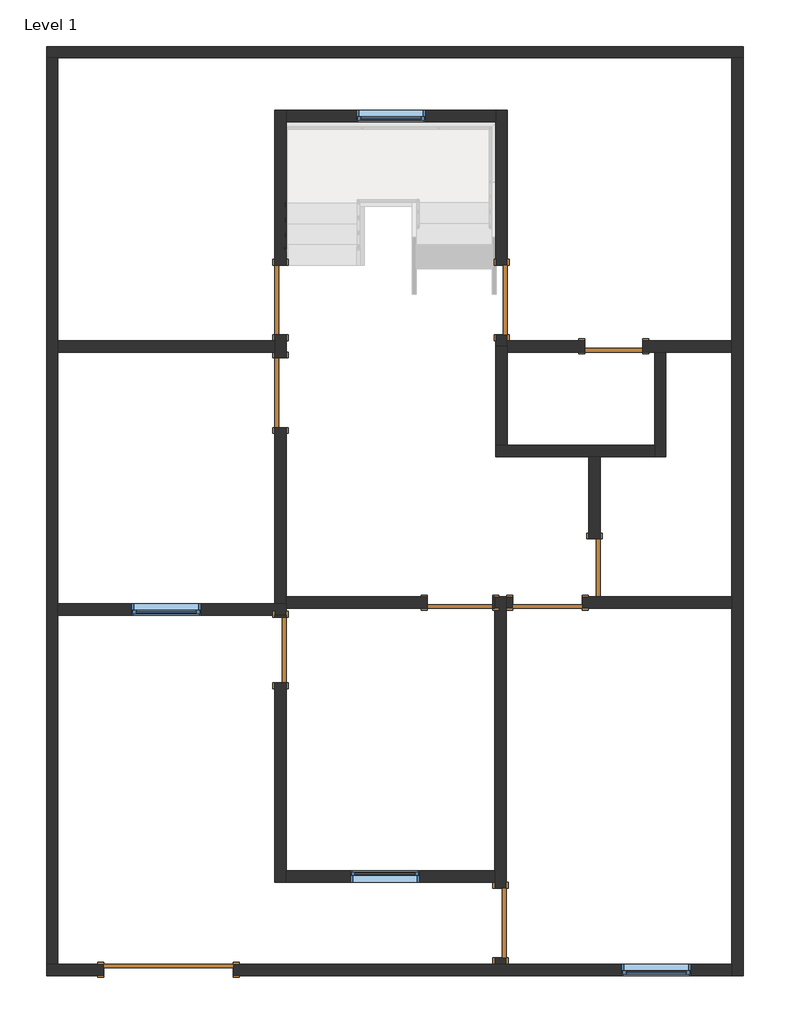
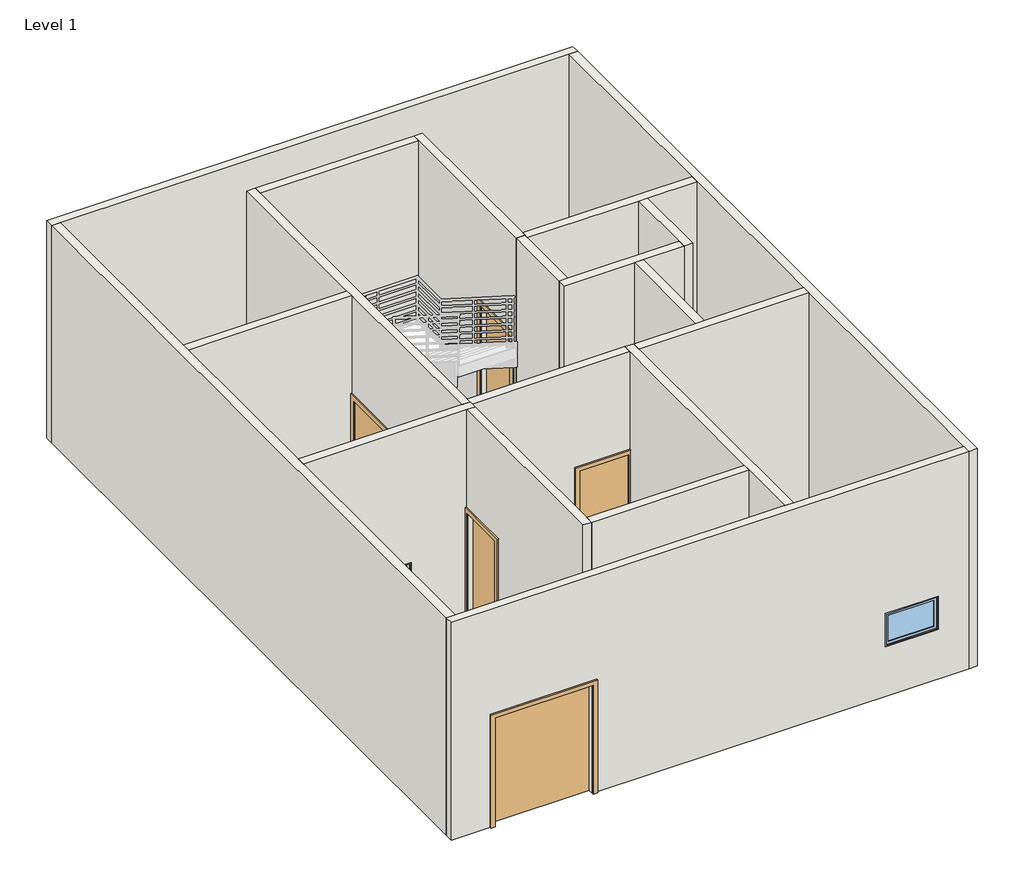
# One storey, part 1 of 3: 19 walls, 10 doors, 4 windows.
"""IFC4 building model written with IfcOpenShell, lengths in millimetres."""

from ifc_helpers import new_model, si_unit, frame, origin, origin_with_axes, place, context, project, spatial, polyline, outline, extrude, faceted_brep, transform, mapped, element, save
from components import m_door_double_flush_panel_double_acting_1700_x_2000mm_42eec5da, m_single_flush_0762_x_2032mm_ffa3ef71, m_single_flush_0762_x_2032mm_3f592dcc, m_single_flush_0864_x_2134mm_0748c0c9, m_single_flush_0915_x_2032mm_d0c19338, m_single_flush_0915_x_2134mm_f3d7f739, m_single_flush_0915_x_2134mm_138fd904, m_fixed_0915_x_0610mm_ad787ded

model = new_model("IFC4")

# Units and contexts
model_context = context("Model", 3, world=origin())
ifc_project = project(units=[si_unit("LENGTHUNIT", "METRE", prefix="MILLI")], contexts=[model_context])

# Site, building, storey
site = spatial("IfcSite", under=ifc_project)
building = spatial("IfcBuilding", under=site)
storey = spatial("IfcBuildingStorey", under=building, Name="Level 1", Elevation=0.0)

# Doors
placement = place(None, origin())
m_door_double_flush_panel_double_acting_1700_x_2000mm_shape = m_door_double_flush_panel_double_acting_1700_x_2000mm_42eec5da(model_context)
element("IfcDoor", 1, ObjectType="M_Door-Double-Flush_Panel-Double-Acting : 1700 x 2000mm", at=placement, inside=storey, context=model_context, shape_type="MappedRepresentation", body=[
    mapped(m_door_double_flush_panel_double_acting_1700_x_2000mm_shape, transform((-12117.6012725, -246.6487671, 0.0), x_axis=(1.0, 0.0, 0.0), y_axis=(0.0, 1.0, 0.0), z_axis=(0.0, 0.0, 1.0))),
])
m_single_flush_0762_x_2032mm_shape = m_single_flush_0762_x_2032mm_ffa3ef71(model_context)
element("IfcDoor", 2, ObjectType="M_Single-Flush : 0762 x 2032mm", at=placement, inside=storey, context=model_context, shape_type="MappedRepresentation", body=[
    mapped(m_single_flush_0762_x_2032mm_shape, transform((-6272.0012725, 7935.7512329, 0.0), x_axis=(1.0, 0.0, 0.0), y_axis=(0.0, 1.0, 0.0), z_axis=(0.0, 0.0, 1.0))),
])
m_single_flush_0762_x_2032mm_2_shape = m_single_flush_0762_x_2032mm_3f592dcc(model_context)
element("IfcDoor", 3, ObjectType="M_Single-Flush : 0762 x 2032mm", at=placement, inside=storey, context=model_context, shape_type="MappedRepresentation", body=[
    mapped(m_single_flush_0762_x_2032mm_2_shape, transform((-6526.0012725, 5028.6512329, 0.0), x_axis=(0.0, -1.0, 0.0), y_axis=(1.0, 0.0, 0.0), z_axis=(0.0, 0.0, 1.0))),
])
m_single_flush_0864_x_2134mm_shape = m_single_flush_0864_x_2134mm_0748c0c9(model_context)
element("IfcDoor", 4, ObjectType="M_Single-Flush : 0864 x 2134mm", at=placement, inside=storey, context=model_context, shape_type="MappedRepresentation", body=[
    mapped(m_single_flush_0864_x_2134mm_shape, transform((-10646.8012725, 3950.3512329, 0.0), x_axis=(0.0, 1.0, 0.0), y_axis=(-1.0, 0.0, 0.0), z_axis=(0.0, 0.0, 1.0))),
])
element("IfcDoor", 5, ObjectType="M_Single-Flush : 0864 x 2134mm", at=placement, inside=storey, context=model_context, shape_type="MappedRepresentation", body=[
    mapped(m_single_flush_0864_x_2134mm_shape, transform((-8290.1012725, 4571.4512329, 0.0), x_axis=(1.0, 0.0, 0.0), y_axis=(0.0, 1.0, 0.0), z_axis=(0.0, 0.0, 1.0))),
])
m_single_flush_0915_x_2032mm_shape = m_single_flush_0915_x_2032mm_d0c19338(model_context)
element("IfcDoor", 6, ObjectType="M_Single-Flush : 0915 x 2032mm", at=placement, inside=storey, context=model_context, shape_type="MappedRepresentation", body=[
    mapped(m_single_flush_0915_x_2032mm_shape, transform((-7141.9512725, 4571.4512329, 0.0), x_axis=(-1.0, 0.0, 0.0), y_axis=(0.0, -1.0, 0.0), z_axis=(0.0, 0.0, 1.0))),
])
element("IfcDoor", 7, ObjectType="M_Single-Flush : 0915 x 2032mm", at=placement, inside=storey, context=model_context, shape_type="MappedRepresentation", body=[
    mapped(m_single_flush_0915_x_2032mm_shape, transform((-7757.9012725, 366.5512329, 0.0), x_axis=(0.0, -1.0, 0.0), y_axis=(1.0, 0.0, 0.0), z_axis=(0.0, 0.0, 1.0))),
])
m_single_flush_0915_x_2134mm_shape = m_single_flush_0915_x_2134mm_f3d7f739(model_context)
element("IfcDoor", 8, ObjectType="M_Single-Flush : 0915 x 2134mm", at=placement, inside=storey, context=model_context, shape_type="MappedRepresentation", body=[
    mapped(m_single_flush_0915_x_2134mm_shape, transform((-10646.8012725, 8545.3512329, 0.0), x_axis=(0.0, -1.0, 0.0), y_axis=(1.0, 0.0, 0.0), z_axis=(0.0, 0.0, 1.0))),
])
m_single_flush_0915_x_2134mm_2_shape = m_single_flush_0915_x_2134mm_138fd904(model_context)
element("IfcDoor", 9, ObjectType="M_Single-Flush : 0915 x 2134mm", at=placement, inside=storey, context=model_context, shape_type="MappedRepresentation", body=[
    mapped(m_single_flush_0915_x_2134mm_2_shape, transform((-7744.0012725, 8545.3512329, 0.0), x_axis=(0.0, -1.0, 0.0), y_axis=(1.0, 0.0, 0.0), z_axis=(0.0, 0.0, 1.0))),
])
element("IfcDoor", 10, ObjectType="M_Single-Flush : 0915 x 2134mm", at=placement, inside=storey, context=model_context, shape_type="MappedRepresentation", body=[
    mapped(m_single_flush_0915_x_2134mm_2_shape, transform((-10646.8012725, 7326.1512329, 0.0), x_axis=(0.0, 1.0, 0.0), y_axis=(-1.0, 0.0, 0.0), z_axis=(0.0, 0.0, 1.0))),
])

# Walls
element("IfcWall", 11, ObjectType="Generic - 150mm", at=placement, inside=storey, context=model_context, shape_type="Brep", body=[
    faceted_brep([(-13716.6012725, 11720.3512329, 0.0), (-13566.6012725, 11720.3512329, 0.0), (-4722.6012725, 11720.3512329, 0.0), (-4572.6012725, 11720.3512329, 0.0), (-4572.6012725, 11720.3512329, 4000.0), (-4722.6012725, 11720.3512329, 4000.0), (-13566.6012725, 11720.3512329, 4000.0), (-13716.6012725, 11720.3512329, 4000.0), (-13716.6012725, 11870.3512329, 0.0), (-13716.6012725, 11870.3512329, 4000.0), (-4572.6012725, 11870.3512329, 4000.0), (-4572.6012725, 11870.3512329, 0.0)], [[[0, 1, 2, 3, 4, 5, 6, 7]], [[8, 9, 10, 11]], [[3, 2, 1, 0, 8, 11]], [[7, 6, 5, 4, 10, 9]], [[4, 3, 11, 10]], [[0, 7, 9, 8]]]),
])
element("IfcWall", 12, ObjectType="Generic - 150mm", at=placement, inside=storey, context=model_context, shape_type="Brep", body=[
    faceted_brep([(-4722.6012725, 11720.3512329, 0.0), (-4722.6012725, 8010.7512329, 0.0), (-4722.6012725, 7860.7512329, 0.0), (-4722.6012725, 4646.4512329, 0.0), (-4722.6012725, 4496.4512329, 0.0), (-4722.6012725, -171.6487671, 0.0), (-4722.6012725, -321.6487671, 0.0), (-4722.6012725, -321.6487671, 4000.0), (-4722.6012725, -171.6487671, 4000.0), (-4722.6012725, 4496.4512329, 4000.0), (-4722.6012725, 4646.4512329, 4000.0), (-4722.6012725, 7860.7512329, 4000.0), (-4722.6012725, 8010.7512329, 4000.0), (-4722.6012725, 11720.3512329, 4000.0), (-4572.6012725, 11720.3512329, 0.0), (-4572.6012725, 11720.3512329, 4000.0), (-4572.6012725, -321.6487671, 4000.0), (-4572.6012725, -321.6487671, 0.0)], [[[0, 1, 2, 3, 4, 5, 6, 7, 8, 9, 10, 11, 12, 13]], [[14, 15, 16, 17]], [[6, 5, 4, 3, 2, 1, 0, 14, 17]], [[13, 12, 11, 10, 9, 8, 7, 16, 15]], [[0, 13, 15, 14]], [[7, 6, 17, 16]]]),
])
element("IfcWall", 13, ObjectType="Generic - 150mm", at=placement, inside=storey, context=model_context, shape_type="Brep", body=[
    faceted_brep([(-13716.6012725, -171.6487671, 4000.0), (-13566.6012725, -171.6487671, 4000.0), (-7832.9012725, -171.6487671, 4000.0), (-7682.9012725, -171.6487671, 4000.0), (-4722.6012725, -171.6487671, 4000.0), (-4722.6012725, -171.6487671, 0.0), (-7682.9012725, -171.6487671, 0.0), (-7832.9012725, -171.6487671, 0.0), (-11267.6012725, -171.6487671, 0.0), (-11267.6012725, -171.6487671, 2000.0), (-12967.6012725, -171.6487671, 2000.0), (-12967.6012725, -171.6487671, 0.0), (-13566.6012725, -171.6487671, 0.0), (-13716.6012725, -171.6487671, 0.0), (-5256.9012725, -171.6487671, 915.0), (-5256.9012725, -171.6487671, 1525.0), (-6171.9012725, -171.6487671, 1525.0), (-6171.9012725, -171.6487671, 915.0), (-4722.6012725, -321.6487671, 4000.0), (-13716.6012725, -321.6487671, 4000.0), (-13716.6012725, -321.6487671, 0.0), (-12967.6012725, -321.6487671, 0.0), (-12967.6012725, -321.6487671, 2000.0), (-11267.6012725, -321.6487671, 2000.0), (-11267.6012725, -321.6487671, 0.0), (-4722.6012725, -321.6487671, 0.0), (-5256.9012725, -321.6487671, 915.0), (-6171.9012725, -321.6487671, 915.0), (-6171.9012725, -321.6487671, 1525.0), (-5256.9012725, -321.6487671, 1525.0)], [[[0, 1, 2, 3, 4, 5, 6, 7, 8, 9, 10, 11, 12, 13], [14, 15, 16, 17]], [[18, 19, 20, 21, 22, 23, 24, 25], [26, 27, 28, 29]], [[5, 25, 24, 8, 7, 6]], [[20, 13, 12, 11, 21]], [[4, 3, 2, 1, 0, 19, 18]], [[5, 4, 18, 25]], [[0, 13, 20, 19]], [[23, 9, 8, 24]], [[9, 23, 22, 10]], [[10, 22, 21, 11]], [[15, 14, 26, 29]], [[16, 15, 29, 28]], [[17, 16, 28, 27]], [[14, 17, 27, 26]]]),
])
element("IfcWall", 14, ObjectType="Generic - 150mm", at=placement, inside=storey, context=model_context, shape_type="Brep", body=[
    faceted_brep([(-13566.6012725, -171.6487671, 0.0), (-13566.6012725, 4407.5512329, 0.0), (-13566.6012725, 4557.5512329, 0.0), (-13566.6012725, 7860.7512329, 0.0), (-13566.6012725, 8010.7512329, 0.0), (-13566.6012725, 11720.3512329, 0.0), (-13566.6012725, 11720.3512329, 4000.0), (-13566.6012725, 8010.7512329, 4000.0), (-13566.6012725, 7860.7512329, 4000.0), (-13566.6012725, 4557.5512329, 4000.0), (-13566.6012725, 4407.5512329, 4000.0), (-13566.6012725, -171.6487671, 4000.0), (-13716.6012725, -171.6487671, 0.0), (-13716.6012725, -171.6487671, 4000.0), (-13716.6012725, 11720.3512329, 4000.0), (-13716.6012725, 11720.3512329, 0.0)], [[[0, 1, 2, 3, 4, 5, 6, 7, 8, 9, 10, 11]], [[12, 13, 14, 15]], [[5, 4, 3, 2, 1, 0, 12, 15]], [[11, 10, 9, 8, 7, 6, 14, 13]], [[6, 5, 15, 14]], [[0, 11, 13, 12]]]),
])
element("IfcWall", 15, ObjectType="Generic - 150mm", at=placement, inside=storey, context=model_context, shape_type="SweptSolid", body=[
    extrude(outline(polyline([(-10721.8012725, 7860.7512329), (-13566.6012725, 7860.7512329), (-13566.6012725, 8010.7512329), (-10721.8012725, 8010.7512329), (-10721.8012725, 7860.7512329)])), origin_with_axes(), (0.0, 0.0, 1.0), 4000.0),
])
element("IfcWall", 16, ObjectType="Generic - 150mm", at=placement, inside=storey, context=model_context, shape_type="Brep", body=[
    faceted_brep([(-10571.8012725, 7783.6512329, 2134.0), (-10571.8012725, 7783.6512329, 0.0), (-10571.8012725, 8087.8512329, 0.0), (-10571.8012725, 8087.8512329, 2134.0), (-10571.8012725, 9002.8512329, 2134.0), (-10571.8012725, 9002.8512329, 0.0), (-10571.8012725, 10883.3512329, 0.0), (-10571.8012725, 11033.3512329, 0.0), (-10571.8012725, 11033.3512329, 4000.0), (-10571.8012725, 10883.3512329, 4000.0), (-10571.8012725, 4646.4512329, 4000.0), (-10571.8012725, 4557.5512329, 4000.0), (-10571.8012725, 4557.5512329, 0.0), (-10571.8012725, 4646.4512329, 0.0), (-10571.8012725, 6868.6512329, 0.0), (-10571.8012725, 6868.6512329, 2134.0), (-10721.8012725, 8087.8512329, 0.0), (-10721.8012725, 8010.7512329, 0.0), (-10721.8012725, 7860.7512329, 0.0), (-10721.8012725, 7783.6512329, 0.0), (-10721.8012725, 7783.6512329, 2134.0), (-10721.8012725, 6868.6512329, 2134.0), (-10721.8012725, 6868.6512329, 0.0), (-10721.8012725, 4557.5512329, 0.0), (-10721.8012725, 4557.5512329, 4000.0), (-10721.8012725, 7860.7512329, 4000.0), (-10721.8012725, 8010.7512329, 4000.0), (-10721.8012725, 11033.3512329, 4000.0), (-10721.8012725, 11033.3512329, 0.0), (-10721.8012725, 9002.8512329, 0.0), (-10721.8012725, 9002.8512329, 2134.0), (-10721.8012725, 8087.8512329, 2134.0)], [[[0, 1, 2, 3, 4, 5, 6, 7, 8, 9, 10, 11, 12, 13, 14, 15]], [[16, 17, 18, 19, 20, 21, 22, 23, 24, 25, 26, 27, 28, 29, 30, 31]], [[29, 28, 7, 6, 5]], [[2, 1, 19, 18, 17, 16]], [[14, 13, 12, 23, 22]], [[11, 10, 9, 8, 27, 26, 25, 24]], [[12, 11, 24, 23]], [[3, 2, 16, 31]], [[4, 3, 31, 30]], [[5, 4, 30, 29]], [[20, 19, 1, 0]], [[21, 20, 0, 15]], [[22, 21, 15, 14]], [[8, 7, 28, 27]]]),
])
element("IfcWall", 17, ObjectType="Generic - 150mm", at=placement, inside=storey, context=model_context, shape_type="Brep", body=[
    faceted_brep([(-4722.6012725, 8010.7512329, 0.0), (-5891.0012725, 8010.7512329, 0.0), (-5891.0012725, 8010.7512329, 2032.0), (-6653.0012725, 8010.7512329, 2032.0), (-6653.0012725, 8010.7512329, 0.0), (-7669.0012725, 8010.7512329, 0.0), (-7669.0012725, 8010.7512329, 4000.0), (-4722.6012725, 8010.7512329, 4000.0), (-5891.0012725, 7860.7512329, 2032.0), (-5891.0012725, 7860.7512329, 0.0), (-5737.4012725, 7860.7512329, 0.0), (-5587.4012725, 7860.7512329, 0.0), (-4722.6012725, 7860.7512329, 0.0), (-4722.6012725, 7860.7512329, 4000.0), (-5587.4012725, 7860.7512329, 4000.0), (-5737.4012725, 7860.7512329, 4000.0), (-7672.6012725, 7860.7512329, 4000.0), (-7672.6012725, 7860.7512329, 0.0), (-6653.0012725, 7860.7512329, 0.0), (-6653.0012725, 7860.7512329, 2032.0), (-7672.6012725, 7935.7512329, 0.0), (-7669.0012725, 7935.7512329, 0.0), (-7669.0012725, 7935.7512329, 4000.0), (-7672.6012725, 7935.7512329, 4000.0)], [[[0, 1, 2, 3, 4, 5, 6, 7]], [[8, 9, 10, 11, 12, 13, 14, 15, 16, 17, 18, 19]], [[18, 17, 20, 21, 5, 4]], [[12, 11, 10, 9, 1, 0]], [[7, 6, 22, 23, 16, 15, 14, 13]], [[0, 7, 13, 12]], [[6, 5, 21, 22]], [[21, 20, 23, 22]], [[20, 17, 16, 23]], [[2, 1, 9, 8]], [[3, 2, 8, 19]], [[4, 3, 19, 18]]]),
])
element("IfcWall", 18, ObjectType="Generic - 150mm", at=placement, inside=storey, context=model_context, shape_type="Brep", body=[
    faceted_brep([(-7669.0012725, 7935.7512329, 0.0), (-7669.0012725, 8010.7512329, 0.0), (-7669.0012725, 8087.8512329, 0.0), (-7669.0012725, 8087.8512329, 2134.0), (-7669.0012725, 9002.8512329, 2134.0), (-7669.0012725, 9002.8512329, 0.0), (-7669.0012725, 11033.3512329, 0.0), (-7669.0012725, 11033.3512329, 4000.0), (-7669.0012725, 8010.7512329, 4000.0), (-7669.0012725, 7935.7512329, 4000.0), (-7819.0012725, 8087.8512329, 2134.0), (-7819.0012725, 8087.8512329, 0.0), (-7819.0012725, 7935.7512329, 0.0), (-7819.0012725, 7935.7512329, 4000.0), (-7819.0012725, 10883.3512329, 4000.0), (-7819.0012725, 11033.3512329, 4000.0), (-7819.0012725, 11033.3512329, 0.0), (-7819.0012725, 10883.3512329, 0.0), (-7819.0012725, 9002.8512329, 0.0), (-7819.0012725, 9002.8512329, 2134.0), (-7672.6012725, 7935.7512329, 0.0), (-7672.6012725, 7935.7512329, 4000.0)], [[[0, 1, 2, 3, 4, 5, 6, 7, 8, 9]], [[10, 11, 12, 13, 14, 15, 16, 17, 18, 19]], [[12, 11, 2, 1, 0, 20]], [[18, 17, 16, 6, 5]], [[9, 8, 7, 15, 14, 13, 21]], [[0, 9, 21, 13, 12, 20]], [[3, 2, 11, 10]], [[4, 3, 10, 19]], [[5, 4, 19, 18]], [[7, 6, 16, 15]]]),
])
element("IfcWall", 19, ObjectType="Generic - 150mm", at=placement, inside=storey, context=model_context, shape_type="Brep", body=[
    faceted_brep([(-13566.6012725, 4407.5512329, 0.0), (-10721.8012725, 4407.5512329, 0.0), (-10571.8012725, 4407.5512329, 0.0), (-10571.8012725, 4407.5512329, 4000.0), (-10721.8012725, 4407.5512329, 4000.0), (-13566.6012725, 4407.5512329, 4000.0), (-11686.7012725, 4407.5512329, 915.0), (-12601.7012725, 4407.5512329, 915.0), (-12601.7012725, 4407.5512329, 1525.0), (-11686.7012725, 4407.5512329, 1525.0), (-13566.6012725, 4557.5512329, 0.0), (-13566.6012725, 4557.5512329, 4000.0), (-10721.8012725, 4557.5512329, 4000.0), (-10571.8012725, 4557.5512329, 4000.0), (-10571.8012725, 4557.5512329, 0.0), (-10721.8012725, 4557.5512329, 0.0), (-11686.7012725, 4557.5512329, 915.0), (-11686.7012725, 4557.5512329, 1525.0), (-12601.7012725, 4557.5512329, 1525.0), (-12601.7012725, 4557.5512329, 915.0), (-10571.8012725, 4496.4512329, 0.0), (-10571.8012725, 4496.4512329, 4000.0)], [[[0, 1, 2, 3, 4, 5], [6, 7, 8, 9]], [[10, 11, 12, 13, 14, 15], [16, 17, 18, 19]], [[2, 1, 0, 10, 15, 14, 20]], [[5, 4, 3, 21, 13, 12, 11]], [[0, 5, 11, 10]], [[3, 2, 20, 14, 13, 21]], [[17, 16, 6, 9]], [[18, 17, 9, 8]], [[19, 18, 8, 7]], [[16, 19, 7, 6]]]),
])
element("IfcWall", 20, ObjectType="Generic - 150mm", at=placement, inside=storey, context=model_context, shape_type="Brep", body=[
    faceted_brep([(-5737.4012725, 7860.7512329, 0.0), (-5737.4012725, 6639.1512329, 0.0), (-5737.4012725, 6489.1512329, 0.0), (-5737.4012725, 6489.1512329, 4000.0), (-5737.4012725, 6639.1512329, 4000.0), (-5737.4012725, 7860.7512329, 4000.0), (-5587.4012725, 7860.7512329, 0.0), (-5587.4012725, 7860.7512329, 4000.0), (-5587.4012725, 6489.1512329, 4000.0), (-5587.4012725, 6489.1512329, 0.0)], [[[0, 1, 2, 3, 4, 5]], [[6, 7, 8, 9]], [[2, 1, 0, 6, 9]], [[5, 4, 3, 8, 7]], [[0, 5, 7, 6]], [[3, 2, 9, 8]]]),
])
element("IfcWall", 21, ObjectType="Generic - 150mm", at=placement, inside=storey, context=model_context, shape_type="Brep", body=[
    faceted_brep([(-5737.4012725, 6639.1512329, 0.0), (-7672.6012725, 6639.1512329, 0.0), (-7822.6012725, 6639.1512329, 0.0), (-7822.6012725, 6639.1512329, 4000.0), (-7672.6012725, 6639.1512329, 4000.0), (-5737.4012725, 6639.1512329, 4000.0), (-5737.4012725, 6489.1512329, 0.0), (-5737.4012725, 6489.1512329, 4000.0), (-6451.0012725, 6489.1512329, 4000.0), (-6601.0012725, 6489.1512329, 4000.0), (-7822.6012725, 6489.1512329, 4000.0), (-7822.6012725, 6489.1512329, 0.0), (-6601.0012725, 6489.1512329, 0.0), (-6451.0012725, 6489.1512329, 0.0)], [[[0, 1, 2, 3, 4, 5]], [[6, 7, 8, 9, 10, 11, 12, 13]], [[2, 1, 0, 6, 13, 12, 11]], [[5, 4, 3, 10, 9, 8, 7]], [[0, 5, 7, 6]], [[3, 2, 11, 10]]]),
])
element("IfcWall", 22, ObjectType="Generic - 150mm", at=placement, inside=storey, context=model_context, shape_type="Brep", body=[
    faceted_brep([(-7672.6012725, 6639.1512329, 0.0), (-7672.6012725, 7860.7512329, 0.0), (-7672.6012725, 7935.7512329, 0.0), (-7672.6012725, 7935.7512329, 4000.0), (-7672.6012725, 7860.7512329, 4000.0), (-7672.6012725, 6639.1512329, 4000.0), (-7822.6012725, 6639.1512329, 0.0), (-7822.6012725, 6639.1512329, 4000.0), (-7822.6012725, 7935.7512329, 4000.0), (-7822.6012725, 7935.7512329, 0.0), (-7819.0012725, 7935.7512329, 0.0), (-7819.0012725, 7935.7512329, 4000.0)], [[[0, 1, 2, 3, 4, 5]], [[6, 7, 8, 9]], [[2, 1, 0, 6, 9, 10]], [[3, 2, 10, 9, 8, 11]], [[5, 4, 3, 11, 8, 7]], [[0, 5, 7, 6]]]),
])
element("IfcWall", 23, ObjectType="Generic - 150mm", at=placement, inside=storey, context=model_context, shape_type="SweptSolid", body=[
    extrude(outline(polyline([(4647.6512329, 2032.0), (4647.6512329, 0.0), (4646.4512329, 0.0), (4646.4512329, 4000.0), (6489.1512329, 4000.0), (6489.1512329, 0.0), (5409.6512329, 0.0), (5409.6512329, 2032.0), (4647.6512329, 2032.0)])), frame((-6601.0012725, 0.0, 0.0), z_axis=(1.0, 0.0, 0.0), x_axis=(0.0, 1.0, 0.0)), (0.0, 0.0, 1.0), 150.0),
])
element("IfcWall", 24, ObjectType="Generic - 150mm", at=placement, inside=storey, context=model_context, shape_type="Brep", body=[
    faceted_brep([(-7682.9012725, 4496.4512329, 0.0), (-7599.4512725, 4496.4512329, 0.0), (-7599.4512725, 4496.4512329, 2032.0), (-6684.4512725, 4496.4512329, 2032.0), (-6684.4512725, 4496.4512329, 0.0), (-4722.6012725, 4496.4512329, 0.0), (-4722.6012725, 4496.4512329, 4000.0), (-7682.9012725, 4496.4512329, 4000.0), (-7599.4512725, 4646.4512329, 2032.0), (-7599.4512725, 4646.4512329, 0.0), (-7682.9012725, 4646.4512329, 0.0), (-7682.9012725, 4646.4512329, 4000.0), (-6601.0012725, 4646.4512329, 4000.0), (-6451.0012725, 4646.4512329, 4000.0), (-4722.6012725, 4646.4512329, 4000.0), (-4722.6012725, 4646.4512329, 0.0), (-6451.0012725, 4646.4512329, 0.0), (-6601.0012725, 4646.4512329, 0.0), (-6684.4512725, 4646.4512329, 0.0), (-6684.4512725, 4646.4512329, 2032.0)], [[[0, 1, 2, 3, 4, 5, 6, 7]], [[8, 9, 10, 11, 12, 13, 14, 15, 16, 17, 18, 19]], [[10, 9, 1, 0]], [[18, 17, 16, 15, 5, 4]], [[7, 6, 14, 13, 12, 11]], [[6, 5, 15, 14]], [[0, 7, 11, 10]], [[2, 1, 9, 8]], [[3, 2, 8, 19]], [[4, 3, 19, 18]]]),
])
element("IfcWall", 25, ObjectType="Generic - 150mm", at=placement, inside=storey, context=model_context, shape_type="Brep", body=[
    faceted_brep([(-7832.9012725, -90.9487671, 2032.0), (-7832.9012725, -90.9487671, 0.0), (-7832.9012725, -171.6487671, 0.0), (-7832.9012725, -171.6487671, 4000.0), (-7832.9012725, 904.7512329, 4000.0), (-7832.9012725, 1054.7512329, 4000.0), (-7832.9012725, 4496.4512329, 4000.0), (-7832.9012725, 4646.4512329, 4000.0), (-7832.9012725, 4646.4512329, 0.0), (-7832.9012725, 4496.4512329, 0.0), (-7832.9012725, 1054.7512329, 0.0), (-7832.9012725, 904.7512329, 0.0), (-7832.9012725, 824.0512329, 0.0), (-7832.9012725, 824.0512329, 2032.0), (-7682.9012725, -171.6487671, 0.0), (-7682.9012725, -90.9487671, 0.0), (-7682.9012725, -90.9487671, 2032.0), (-7682.9012725, 824.0512329, 2032.0), (-7682.9012725, 824.0512329, 0.0), (-7682.9012725, 4496.4512329, 0.0), (-7682.9012725, 4646.4512329, 0.0), (-7682.9012725, 4646.4512329, 4000.0), (-7682.9012725, 4496.4512329, 4000.0), (-7682.9012725, -171.6487671, 4000.0)], [[[0, 1, 2, 3, 4, 5, 6, 7, 8, 9, 10, 11, 12, 13]], [[14, 15, 16, 17, 18, 19, 20, 21, 22, 23]], [[2, 1, 15, 14]], [[12, 11, 10, 9, 8, 20, 19, 18]], [[7, 6, 5, 4, 3, 23, 22, 21]], [[3, 2, 14, 23]], [[8, 7, 21, 20]], [[16, 15, 1, 0]], [[17, 16, 0, 13]], [[18, 17, 13, 12]]]),
])
element("IfcWall", 26, ObjectType="Generic - 150mm", at=placement, inside=storey, context=model_context, shape_type="Brep", body=[
    faceted_brep([(-10721.8012725, 4407.5512329, 0.0), (-10721.8012725, 4382.3512329, 0.0), (-10721.8012725, 4382.3512329, 2134.0), (-10721.8012725, 3518.3512329, 2134.0), (-10721.8012725, 3518.3512329, 0.0), (-10721.8012725, 904.7512329, 0.0), (-10721.8012725, 904.7512329, 4000.0), (-10721.8012725, 4407.5512329, 4000.0), (-10571.8012725, 4382.3512329, 2134.0), (-10571.8012725, 4382.3512329, 0.0), (-10571.8012725, 4407.5512329, 0.0), (-10571.8012725, 4407.5512329, 4000.0), (-10571.8012725, 1054.7512329, 4000.0), (-10571.8012725, 904.7512329, 4000.0), (-10571.8012725, 904.7512329, 0.0), (-10571.8012725, 1054.7512329, 0.0), (-10571.8012725, 3518.3512329, 0.0), (-10571.8012725, 3518.3512329, 2134.0)], [[[0, 1, 2, 3, 4, 5, 6, 7]], [[8, 9, 10, 11, 12, 13, 14, 15, 16, 17]], [[10, 9, 1, 0]], [[16, 15, 14, 5, 4]], [[7, 6, 13, 12, 11]], [[0, 7, 11, 10]], [[6, 5, 14, 13]], [[2, 1, 9, 8]], [[3, 2, 8, 17]], [[4, 3, 17, 16]]]),
])
element("IfcWall", 27, ObjectType="Generic - 150mm", at=placement, inside=storey, context=model_context, shape_type="SweptSolid", body=[
    extrude(outline(polyline([(0.0, -10571.8012725), (0.0, -7832.9012725), (4000.0, -7832.9012725), (4000.0, -10571.8012725), (0.0, -10571.8012725)]), holes=[polyline([(915.0, -9732.7012725), (1525.0, -9732.7012725), (1525.0, -8817.7012725), (915.0, -8817.7012725), (915.0, -9732.7012725)])]), frame((0.0, 904.7512329, 0.0), z_axis=(0.0, 1.0, 0.0), x_axis=(0.0, 0.0, 1.0)), (0.0, 0.0, 1.0), 150.0),
])
element("IfcWall", 28, ObjectType="Generic - 150mm", at=placement, inside=storey, context=model_context, shape_type="Brep", body=[
    faceted_brep([(-7832.9012725, 4646.4512329, 0.0), (-7858.1012725, 4646.4512329, 0.0), (-7858.1012725, 4646.4512329, 2134.0), (-8722.1012725, 4646.4512329, 2134.0), (-8722.1012725, 4646.4512329, 0.0), (-10571.8012725, 4646.4512329, 0.0), (-10571.8012725, 4646.4512329, 4000.0), (-7832.9012725, 4646.4512329, 4000.0), (-7858.1012725, 4496.4512329, 2134.0), (-7858.1012725, 4496.4512329, 0.0), (-7832.9012725, 4496.4512329, 0.0), (-7832.9012725, 4496.4512329, 4000.0), (-10571.8012725, 4496.4512329, 4000.0), (-10571.8012725, 4496.4512329, 0.0), (-8722.1012725, 4496.4512329, 0.0), (-8722.1012725, 4496.4512329, 2134.0), (-10571.8012725, 4557.5512329, 0.0), (-10571.8012725, 4557.5512329, 4000.0)], [[[0, 1, 2, 3, 4, 5, 6, 7]], [[8, 9, 10, 11, 12, 13, 14, 15]], [[14, 13, 16, 5, 4]], [[10, 9, 1, 0]], [[7, 6, 17, 12, 11]], [[0, 7, 11, 10]], [[6, 5, 16, 13, 12, 17]], [[2, 1, 9, 8]], [[3, 2, 8, 15]], [[4, 3, 15, 14]]]),
])
element("IfcWall", 29, ObjectType="Generic - 150mm", at=placement, inside=storey, context=model_context, shape_type="SweptSolid", body=[
    extrude(outline(polyline([(0.0, -10571.8012725), (0.0, -7819.0012725), (4000.0, -7819.0012725), (4000.0, -10571.8012725), (0.0, -10571.8012725)]), holes=[polyline([(915.0, -8737.9012725), (915.0, -9652.9012725), (1525.0, -9652.9012725), (1525.0, -8737.9012725), (915.0, -8737.9012725)])]), frame((0.0, 10883.3512329, 0.0), z_axis=(0.0, 1.0, 0.0), x_axis=(0.0, 0.0, 1.0)), (0.0, 0.0, 1.0), 150.0),
])

# Windows
m_fixed_0915_x_0610mm_shape = m_fixed_0915_x_0610mm_ad787ded(model_context)
element("IfcWindow", 30, ObjectType="M_Fixed : 0915 x 0610mm", at=placement, inside=storey, context=model_context, shape_type="MappedRepresentation", body=[
    mapped(m_fixed_0915_x_0610mm_shape, transform((-9275.2012725, 966.7512329, 0.0), x_axis=(1.0, 0.0, 0.0), y_axis=(0.0, 1.0, 0.0), z_axis=(0.0, 0.0, 1.0))),
])
element("IfcWindow", 31, ObjectType="M_Fixed : 0915 x 0610mm", at=placement, inside=storey, context=model_context, shape_type="MappedRepresentation", body=[
    mapped(m_fixed_0915_x_0610mm_shape, transform((-12144.2012725, 4495.5512329, 0.0), x_axis=(-1.0, 0.0, 0.0), y_axis=(0.0, -1.0, 0.0), z_axis=(0.0, 0.0, 1.0))),
])
element("IfcWindow", 32, ObjectType="M_Fixed : 0915 x 0610mm", at=placement, inside=storey, context=model_context, shape_type="MappedRepresentation", body=[
    mapped(m_fixed_0915_x_0610mm_shape, transform((-9195.4012725, 10971.3512329, 0.0), x_axis=(-1.0, 0.0, 0.0), y_axis=(0.0, -1.0, 0.0), z_axis=(0.0, 0.0, 1.0))),
])
element("IfcWindow", 33, ObjectType="M_Fixed : 0915 x 0610mm", at=placement, inside=storey, context=model_context, shape_type="MappedRepresentation", body=[
    mapped(m_fixed_0915_x_0610mm_shape, transform((-5714.4012725, -233.6487671, 0.0), x_axis=(-1.0, 0.0, 0.0), y_axis=(0.0, -1.0, 0.0), z_axis=(0.0, 0.0, 1.0))),
])

save(model, "model.ifc")

# Revit data of these elements
# Type "M_Door-Double-Flush_Panel-Double-Acting : 1700 x 2000mm"
#   Type Mark = "22"
#   Construction Type Id = "DOOR"
#   Assembly Code = "C1020"
#   Analytic Construction = "Wooden"
#   W = 850 mm
#   Thickness = 50 mm
#   Thermal Resistance (R) = 0.455703 (m²·K)/W
#   Swing Angle [instance default] = 90.00°
#   Heat Transfer Coefficient (U) = 2.19465 W/(m²·K)
#   Height = 2000 mm
#   Trim Projection Ext. = 25 mm
#   Trim Projection Int. = 25 mm
#   Trim Width Ext. = 80 mm
#   Trim Width Int. = 80 mm
#   Width = 1700 mm
#   Define Thermal Properties by = 1
#   Panel Material = Wood - Birch - Solid Stained Light Low Gloss
#   Trim Material = Paint - Sienna
#   Visual Light Transmittance = 0
#   Solar Heat Gain Coefficient = 0
#   Function = (empty or 0)
#   Wall Closure = (empty or 0)
# Type "M_Single-Flush : 0762 x 2032mm"
#   Type Mark = "19"
#   Thickness = 51 mm
#   Height = 2032 mm
#   Trim Projection Ext = 25 mm
#   Trim Projection Int = 25 mm
#   Trim Width = 76 mm
#   Width = 762 mm
#   Door Material = Door - Panel
#   Frame Material = Door - Frame
#   Function = (empty or 0)
#   Wall Closure = (empty or 0)
# Type "M_Single-Flush : 0864 x 2134mm"
#   Type Mark = "16"
#   Thickness = 51 mm
#   Height = 2134 mm
#   Trim Projection Ext = 25 mm
#   Trim Projection Int = 25 mm
#   Trim Width = 76 mm
#   Width = 864 mm
#   Door Material = Door - Panel
#   Frame Material = Door - Frame
#   Function = (empty or 0)
#   Wall Closure = (empty or 0)
# Type "M_Single-Flush : 0915 x 2032mm"
#   Type Mark = "20"
#   Thickness = 51 mm
#   Height = 2032 mm
#   Trim Projection Ext = 25 mm
#   Trim Projection Int = 25 mm
#   Trim Width = 76 mm
#   Width = 915 mm
#   Door Material = Door - Panel
#   Frame Material = Door - Frame
#   Function = (empty or 0)
#   Wall Closure = (empty or 0)
# Type "M_Single-Flush : 0915 x 2134mm"
#   Type Mark = "15"
#   Thickness = 51 mm
#   Height = 2134 mm
#   Trim Projection Ext = 25 mm
#   Trim Projection Int = 25 mm
#   Trim Width = 76 mm
#   Width = 915 mm
#   Door Material = Door - Panel
#   Frame Material = Door - Frame
#   Function = (empty or 0)
#   Wall Closure = (empty or 0)
# Type "Generic - 150mm"
#   Layers, outside or top first: 150 mm no material (function 1)
# Type "M_Fixed : 0915 x 0610mm"
#   Type Mark = "14"
#   Height = 610 mm
#   Default Sill Height = 915 mm
#   Width = 915 mm
#   Window Inset = 19 mm
#   Frame Exterior Material = Sash
#   Frame Interior Material = Sash
#   Glass Pane Material = Glass
#   Sash = Sash
#   Wall Closure = (empty or 0)
# Element 1 (IfcDoor, "M_Door-Double-Flush_Panel-Double-Acting : 1700 x 2000mm")
#   Swing Angle = 90.00°
#   Phase Created = New Construction
#   Materials on its faces: "Paint - Sienna", "Wood - Birch - Solid Stained Light Low Gloss"
# Elements 2, 3 (IfcDoor, "M_Single-Flush : 0762 x 2032mm")
#   Phase Created = New Construction
#   Materials on its faces: "Door - Frame", "Door - Panel"
# Elements 4, 5 (IfcDoor, "M_Single-Flush : 0864 x 2134mm")
#   Phase Created = New Construction
#   Materials on its faces: "Door - Frame", "Door - Panel"
# Elements 6, 7 (IfcDoor, "M_Single-Flush : 0915 x 2032mm")
#   Phase Created = New Construction
#   Materials on its faces: "Door - Frame", "Door - Panel"
# Elements 8, 9, 10 (IfcDoor, "M_Single-Flush : 0915 x 2134mm")
#   Phase Created = New Construction
#   Materials on its faces: "Door - Frame", "Door - Panel"
# Elements 11, 12, 13, 14, 15, 16, 17, 18, 19, 20, 21, 22, 23, 24, 25, 26, 27, 28, 29 (IfcWall, "Generic - 150mm")
#   Top Offset = 0 mm
#   Base Offset = 0 mm
#   wall height = 4000 mm
#   Phase Created = New Construction
#   Base Constraint = Level 1
#   Top Constraint = Level 2
#   Materials on its faces: "Default Wall"
# Element 30 (IfcWindow, "M_Fixed : 0915 x 0610mm")
#   Mark = "6"
#   Phase Created = New Construction
#   Materials on its faces: "Sash", "Glass"
# Element 31 (IfcWindow, "M_Fixed : 0915 x 0610mm")
#   Mark = "7"
#   Phase Created = New Construction
#   Materials on its faces: "Sash", "Glass"
# Element 32 (IfcWindow, "M_Fixed : 0915 x 0610mm")
#   Mark = "8"
#   Phase Created = New Construction
#   Materials on its faces: "Sash", "Glass"
# Element 33 (IfcWindow, "M_Fixed : 0915 x 0610mm")
#   Mark = "9"
#   Phase Created = New Construction
#   Materials on its faces: "Sash", "Glass"
# Materials
#   "Wood - Birch - Solid Stained Light Low Gloss": class "Wood", colour RGB 210 159 95, transparency 0, Cost = 0
#   "Paint - Sienna": colour RGB 118 70 51, transparency 0, Cost = 0
#   "Door - Panel": class "Wood", colour RGB 114 82 51, transparency 0
#   "Door - Frame": colour RGB 153 76 43, transparency 0
#   "Sash": class "Wood", colour RGB 136 99 55, transparency 0
#   "Glass": class "Glass", colour RGB 218 227 224, transparency 0.85, Description = "Soda Lime Glass", Cost = 0
#   "Default Wall": colour RGB 80 80 80, transparency 0
